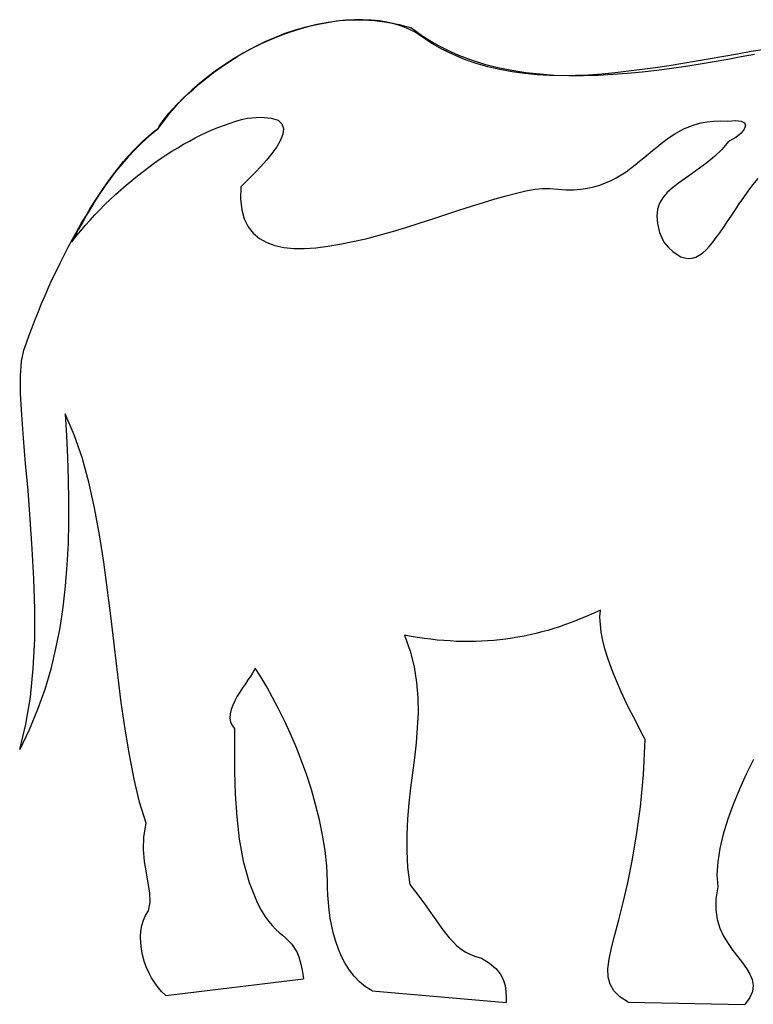
# Model space of a CAD drawing. Units: inches. Extents: x 386 to 107067, y -7 to 96314.
# Tile 7 of 10: x 101861.777 to 101863.94, y 96247.493 to 96250.395. Entities that reach past the tile are written whole.
import ezdxf

# ---------------------------------------------------------------- set-up
doc = ezdxf.new("R2010")
doc.units = ezdxf.units.IN
doc.layers.add('A-ELEV', color=7, linetype='Continuous', lineweight=25)
doc.layers.add('freecads.com', color=7, linetype='Continuous')

# ---------------------------------------------------------------- blocks, each defined once
blk = doc.blocks.new('elephant')
at = {"layer": 'freecads.com'}
for p, q in [((104457.3165, 95264.9791), (104457.3504, 95264.9835)), ((104457.3684, 95264.9845), (104457.3416, 95264.9818)), ((104457.3504, 95264.9835), (104457.3843, 95264.9856)), ((104457.3941, 95264.9862), (104457.3684, 95264.9845)), ((104457.3843, 95264.9856), (104457.4193, 95264.9856)), ((104457.4193, 95264.9862), (104457.3941, 95264.9862)), ((104457.4439, 95264.9851), (104457.4193, 95264.9862)), ((104457.4193, 95264.9856), (104457.4543, 95264.9835)), ((104457.4674, 95264.9829), (104457.4439, 95264.9851)), ((104457.4543, 95264.9835), (104457.4898, 95264.9791)), ((104457.4898, 95264.9791), (104457.4674, 95264.9829)), ((104457.1896, 95264.9463), (104457.2202, 95264.9567)), ((104457.2328, 95264.9583), (104457.2049, 95264.949)), ((104457.2202, 95264.9567), (104457.2514, 95264.9654)), ((104457.2601, 95264.966), (104457.2328, 95264.9583)), ((104457.2514, 95264.9654), (104457.2836, 95264.9731)), ((104457.288, 95264.9725), (104457.2601, 95264.966)), ((104457.2836, 95264.9731), (104457.3165, 95264.9791)), ((104457.3148, 95264.9774), (104457.288, 95264.9725)), ((104457.3416, 95264.9818), (104457.3148, 95264.9774)), ((104457.4898, 95264.9791), (104457.5259, 95264.972)), ((104457.5117, 95264.9742), (104457.4898, 95264.9791)), ((104457.5325, 95264.9676), (104457.5117, 95264.9742)), ((104457.5259, 95264.972), (104457.5625, 95264.9621)), ((104457.5522, 95264.9594), (104457.5325, 95264.9676)), ((104457.5708, 95264.9501), (104457.5522, 95264.9594)), ((104457.5625, 95264.9621), (104457.5954, 95264.9381)), ((104457.1491, 95264.9277), (104457.1212, 95264.9156)), ((104457.1311, 95264.9217), (104457.1595, 95264.9342)), ((104457.177, 95264.9392), (104457.1491, 95264.9277)), ((104457.1595, 95264.9342), (104457.1896, 95264.9463)), ((104457.2049, 95264.949), (104457.177, 95264.9392)), ((104457.5877, 95264.9392), (104457.5708, 95264.9501)), ((104457.6194, 95264.9184), (104457.5877, 95264.9392)), ((104457.5954, 95264.9381), (104457.6292, 95264.9167)), ((104457.0939, 95264.902), (104457.0665, 95264.8872)), ((104457.0758, 95264.8932), (104457.1032, 95264.908)), ((104457.1212, 95264.9156), (104457.0939, 95264.902)), ((104457.1032, 95264.908), (104457.1311, 95264.9217)), ((104457.6517, 95264.8998), (104457.6194, 95264.9184)), ((104457.6292, 95264.9167), (104457.6648, 95264.8981)), ((104457.685, 95264.8834), (104457.6517, 95264.8998)), ((104457.6648, 95264.8981), (104457.7009, 95264.8817)), ((104458.6048, 95264.8987), (104458.5644, 95264.8921)), ((104457.0398, 95264.8719), (104457.0135, 95264.8549)), ((104457.0255, 95264.8626), (104457.0501, 95264.8784)), ((104457.0665, 95264.8872), (104457.0398, 95264.8719)), ((104457.0501, 95264.8784), (104457.0758, 95264.8932)), ((104457.7184, 95264.8691), (104457.685, 95264.8834)), ((104457.7009, 95264.8817), (104457.7386, 95264.8675)), ((104457.7528, 95264.8571), (104457.7184, 95264.8691)), ((104457.7386, 95264.8675), (104457.7775, 95264.8555)), ((104458.443, 95264.8708), (104458.4025, 95264.8642)), ((104458.4834, 95264.8779), (104458.443, 95264.8708)), ((104458.4545, 95264.8631), (104458.4949, 95264.8702)), ((104458.5239, 95264.885), (104458.4834, 95264.8779)), ((104458.4949, 95264.8702), (104458.5348, 95264.8773)), ((104458.5644, 95264.8921), (104458.5239, 95264.885)), ((104458.5348, 95264.8773), (104458.5737, 95264.885)), ((104456.9878, 95264.8374), (104456.9626, 95264.8189)), ((104456.979, 95264.8303), (104457.0015, 95264.8467)), ((104457.0135, 95264.8549), (104456.9878, 95264.8374)), ((104457.0015, 95264.8467), (104457.0255, 95264.8626)), ((104457.7878, 95264.8473), (104457.7528, 95264.8571)), ((104457.7775, 95264.8555), (104457.8174, 95264.8451)), ((104457.8234, 95264.8391), (104457.7878, 95264.8473)), ((104457.8174, 95264.8451), (104457.8579, 95264.8374)), ((104457.8595, 95264.8325), (104457.8234, 95264.8391)), ((104457.8579, 95264.8374), (104457.8994, 95264.8309)), ((104458.2423, 95264.8391), (104458.2024, 95264.8342)), ((104458.2822, 95264.8446), (104458.2423, 95264.8391)), ((104458.2429, 95264.8325), (104458.286, 95264.8374)), ((104458.3221, 95264.8506), (104458.2822, 95264.8446)), ((104458.286, 95264.8374), (104458.3287, 95264.8435)), ((104458.3621, 95264.8571), (104458.3221, 95264.8506)), ((104458.3287, 95264.8435), (104458.3714, 95264.8495)), ((104458.4025, 95264.8642), (104458.3621, 95264.8571)), ((104458.3714, 95264.8495), (104458.4135, 95264.856)), ((104458.4135, 95264.856), (104458.4545, 95264.8631)), ((104456.9626, 95264.8189), (104456.938, 95264.7992)), ((104456.938, 95264.7981), (104456.9577, 95264.8139)), ((104456.9577, 95264.8139), (104456.979, 95264.8303)), ((104457.8961, 95264.8276), (104457.8595, 95264.8325)), ((104457.9328, 95264.8238), (104457.8961, 95264.8276)), ((104457.8994, 95264.8309), (104457.941, 95264.8265)), ((104457.9705, 95264.8221), (104457.9328, 95264.8238)), ((104457.941, 95264.8265), (104457.9836, 95264.8232)), ((104458.0082, 95264.821), (104457.9705, 95264.8221)), ((104457.9836, 95264.8232), (104458.0263, 95264.8221)), ((104458.0465, 95264.8216), (104458.0082, 95264.821)), ((104458.0263, 95264.8221), (104458.0695, 95264.8221)), ((104458.0848, 95264.8232), (104458.0465, 95264.8216)), ((104458.0695, 95264.8221), (104458.1127, 95264.8232)), ((104458.1236, 95264.826), (104458.0848, 95264.8232)), ((104458.1127, 95264.8232), (104458.1559, 95264.8254)), ((104458.163, 95264.8298), (104458.1236, 95264.826)), ((104458.1559, 95264.8254), (104458.1996, 95264.8287)), ((104458.2024, 95264.8342), (104458.163, 95264.8298)), ((104458.1996, 95264.8287), (104458.2429, 95264.8325)), ((104456.9019, 95264.7663), (104456.9194, 95264.7817)), ((104456.938, 95264.7992), (104456.9145, 95264.7784)), ((104456.9194, 95264.7817), (104456.938, 95264.7981)), ((104456.8915, 95264.757), (104456.8697, 95264.7341)), ((104456.8719, 95264.7368), (104456.8861, 95264.751)), ((104456.8861, 95264.751), (104456.9019, 95264.7663)), ((104456.9145, 95264.7784), (104456.8915, 95264.757)), ((104456.8472, 95264.7106), (104456.8587, 95264.7231)), ((104456.8697, 95264.7341), (104456.8489, 95264.7111)), ((104456.8587, 95264.7231), (104456.8719, 95264.7368)), ((104456.8489, 95264.7111), (104456.8297, 95264.6865)), ((104456.8297, 95264.6887), (104456.8379, 95264.6985)), ((104456.8379, 95264.6985), (104456.8472, 95264.7106)), ((104457.0447, 95264.6871), (104457.0616, 95264.692)), ((104457.0616, 95264.692), (104457.078, 95264.6958)), ((104457.078, 95264.6958), (104457.1185, 95264.6985)), ((104457.1185, 95264.6985), (104457.1486, 95264.6964)), ((104457.1486, 95264.6964), (104457.1688, 95264.6898)), ((104456.8013, 95264.6553), (104456.8161, 95264.6663)), ((104456.8297, 95264.6865), (104456.8111, 95264.6613)), ((104456.8161, 95264.6663), (104456.8188, 95264.6723)), ((104456.8188, 95264.6723), (104456.8232, 95264.6794)), ((104456.8232, 95264.6794), (104456.8297, 95264.6887)), ((104456.9768, 95264.6624), (104456.9938, 95264.6696)), ((104456.9938, 95264.6696), (104457.0108, 95264.6756)), ((104457.0108, 95264.6756), (104457.0277, 95264.6816)), ((104457.0277, 95264.6816), (104457.0447, 95264.6871)), ((104457.1688, 95264.6898), (104457.1803, 95264.6794)), ((104457.1803, 95264.6794), (104457.1852, 95264.6652)), ((104457.1852, 95264.6652), (104457.183, 95264.6493)), ((104458.3528, 95264.6581), (104458.3675, 95264.6652)), ((104458.3675, 95264.6652), (104458.3828, 95264.6717)), ((104458.3828, 95264.6717), (104458.3993, 95264.6778)), ((104458.3993, 95264.6778), (104458.4162, 95264.6821)), ((104458.4162, 95264.6821), (104458.4342, 95264.6854)), ((104458.4342, 95264.6854), (104458.4534, 95264.6876)), ((104458.4534, 95264.6876), (104458.473, 95264.6882)), ((104458.473, 95264.6882), (104458.4944, 95264.6871)), ((104458.4944, 95264.6871), (104458.5184, 95264.6892)), ((104458.5184, 95264.6892), (104458.5348, 95264.6876)), ((104458.5436, 95264.6635), (104458.5343, 95264.652)), ((104458.5348, 95264.6876), (104458.5447, 95264.6821)), ((104458.5474, 95264.6739), (104458.5436, 95264.6635)), ((104458.5447, 95264.6821), (104458.5474, 95264.6739)), ((104456.7887, 95264.6428), (104456.7669, 95264.6231)), ((104456.7718, 95264.6302), (104456.7865, 95264.6433)), ((104456.7865, 95264.6433), (104456.8013, 95264.6553)), ((104456.8111, 95264.6613), (104456.7887, 95264.6428)), ((104456.9074, 95264.6285), (104456.9249, 95264.6378)), ((104456.9249, 95264.6378), (104456.9424, 95264.6466)), ((104456.9424, 95264.6466), (104456.9593, 95264.6548)), ((104456.9593, 95264.6548), (104456.9768, 95264.6624)), ((104457.183, 95264.6493), (104457.1765, 95264.6313)), ((104458.3117, 95264.6313), (104458.3249, 95264.6411)), ((104458.3249, 95264.6411), (104458.3385, 95264.6499)), ((104458.3385, 95264.6499), (104458.3528, 95264.6581)), ((104458.5184, 95264.6395), (104458.4977, 95264.6274)), ((104458.5343, 95264.652), (104458.5184, 95264.6395)), ((104456.7422, 95264.6012), (104456.757, 95264.6159)), ((104456.7669, 95264.6231), (104456.7466, 95264.6028)), ((104456.757, 95264.6159), (104456.7718, 95264.6302)), ((104456.8554, 95264.5985), (104456.8729, 95264.6088)), ((104456.8729, 95264.6088), (104456.8905, 95264.6192)), ((104456.8905, 95264.6192), (104456.9074, 95264.6285)), ((104457.165, 95264.6116), (104457.1508, 95264.5919)), ((104457.1765, 95264.6313), (104457.165, 95264.6116)), ((104458.2729, 95264.6006), (104458.2855, 95264.611)), ((104458.2855, 95264.611), (104458.2986, 95264.6214)), ((104458.2986, 95264.6214), (104458.3117, 95264.6313)), ((104458.4977, 95264.6274), (104458.4774, 95264.6039)), ((104456.7269, 95264.5821), (104456.7083, 95264.5607)), ((104456.7133, 95264.5684), (104456.728, 95264.5848)), ((104456.7466, 95264.6028), (104456.7269, 95264.5821)), ((104456.728, 95264.5848), (104456.7422, 95264.6012)), ((104456.8046, 95264.564), (104456.8215, 95264.576)), ((104456.8215, 95264.576), (104456.8385, 95264.5875)), ((104456.8385, 95264.5875), (104456.8554, 95264.5985)), ((104457.1508, 95264.5919), (104457.1349, 95264.5722)), ((104458.2352, 95264.5689), (104458.2478, 95264.5793)), ((104458.2478, 95264.5793), (104458.2604, 95264.5903)), ((104458.2604, 95264.5903), (104458.2729, 95264.6006)), ((104458.4561, 95264.5831), (104458.4337, 95264.5646)), ((104458.4774, 95264.6039), (104458.4561, 95264.5831)), ((104456.6848, 95264.5317), (104456.699, 95264.5503)), ((104456.7083, 95264.5607), (104456.6908, 95264.5394)), ((104456.699, 95264.5503), (104456.7133, 95264.5684)), ((104456.7707, 95264.5389), (104456.7876, 95264.5514)), ((104456.7876, 95264.5514), (104456.8046, 95264.564)), ((104457.1179, 95264.5531), (104457.1015, 95264.5361)), ((104457.1349, 95264.5722), (104457.1179, 95264.5531)), ((104458.1953, 95264.5383), (104458.2089, 95264.5482)), ((104458.2089, 95264.5482), (104458.2221, 95264.5585)), ((104458.2221, 95264.5585), (104458.2352, 95264.5689)), ((104458.4118, 95264.5482), (104458.3905, 95264.5328)), ((104458.4337, 95264.5646), (104458.4118, 95264.5482)), ((104456.6701, 95264.5126), (104456.6848, 95264.5317)), ((104456.6908, 95264.5394), (104456.6739, 95264.5175)), ((104456.7379, 95264.5126), (104456.7543, 95264.5263)), ((104456.7543, 95264.5263), (104456.7707, 95264.5389)), ((104457.0862, 95264.5208), (104457.0736, 95264.5082)), ((104457.1015, 95264.5361), (104457.0862, 95264.5208)), ((104458.151, 95264.5126), (104458.1663, 95264.5203)), ((104458.1663, 95264.5203), (104458.181, 95264.529)), ((104458.181, 95264.529), (104458.1953, 95264.5383)), ((104458.3697, 95264.5186), (104458.35, 95264.5044)), ((104458.3905, 95264.5328), (104458.3697, 95264.5186)), ((104458.5693, 95264.4995), (104458.5846, 95264.5181)), ((104456.6422, 95264.4721), (104456.6564, 95264.4929)), ((104456.658, 95264.4956), (104456.6433, 95264.4738)), ((104456.6564, 95264.4929), (104456.6701, 95264.5126)), ((104456.6739, 95264.5175), (104456.658, 95264.4956)), ((104456.7056, 95264.4852), (104456.7215, 95264.4989)), ((104456.7215, 95264.4989), (104456.7379, 95264.5126)), ((104457.0594, 95264.494), (104457.0583, 95264.4579)), ((104457.0643, 95264.4989), (104457.0594, 95264.494)), ((104457.0736, 95264.5082), (104457.0643, 95264.4989)), ((104457.9257, 95264.4863), (104457.9486, 95264.4891)), ((104457.9486, 95264.4891), (104457.9689, 95264.4891)), ((104457.9689, 95264.4891), (104457.994, 95264.4863)), ((104458.0613, 95264.4863), (104458.081, 95264.4896)), ((104458.081, 95264.4896), (104458.1001, 95264.4935)), ((104458.1001, 95264.4935), (104458.1176, 95264.4989)), ((104458.1176, 95264.4989), (104458.1346, 95264.5055)), ((104458.1346, 95264.5055), (104458.151, 95264.5126)), ((104458.3325, 95264.4907), (104458.3167, 95264.4765)), ((104458.35, 95264.5044), (104458.3325, 95264.4907)), ((104458.5551, 95264.4809), (104458.5693, 95264.4995)), ((104456.6285, 95264.4513), (104456.6422, 95264.4721)), ((104456.6433, 95264.4738), (104456.6291, 95264.4519)), ((104456.6739, 95264.4563), (104456.6897, 95264.471)), ((104456.6897, 95264.471), (104456.7056, 95264.4852)), ((104457.8092, 95264.4579), (104457.8415, 95264.4672)), ((104457.8415, 95264.4672), (104457.8721, 95264.4754)), ((104457.8721, 95264.4754), (104457.8999, 95264.482)), ((104457.8999, 95264.482), (104457.9257, 95264.4863)), ((104457.994, 95264.4863), (104458.0175, 95264.4847)), ((104458.0175, 95264.4847), (104458.0399, 95264.4847)), ((104458.0399, 95264.4847), (104458.0613, 95264.4863)), ((104458.3035, 95264.4617), (104458.2937, 95264.4459)), ((104458.3167, 95264.4765), (104458.3035, 95264.4617)), ((104458.5288, 95264.4437), (104458.542, 95264.4623)), ((104458.542, 95264.4623), (104458.5551, 95264.4809)), ((104456.6148, 95264.4295), (104456.6285, 95264.4513)), ((104456.6291, 95264.4519), (104456.6159, 95264.43)), ((104456.6438, 95264.4262), (104456.6586, 95264.4415)), ((104456.6586, 95264.4415), (104456.6739, 95264.4563)), ((104457.0583, 95264.4579), (104457.0622, 95264.4262)), ((104457.702, 95264.4246), (104457.7392, 95264.4366)), ((104457.7392, 95264.4366), (104457.7747, 95264.4475)), ((104457.7747, 95264.4475), (104457.8092, 95264.4579)), ((104458.2937, 95264.4459), (104458.2877, 95264.4278)), ((104458.5168, 95264.4251), (104458.5288, 95264.4437)), ((104456.5886, 95264.3852), (104456.6017, 95264.4076)), ((104456.6033, 95264.4092), (104456.5919, 95264.3885)), ((104456.6017, 95264.4076), (104456.6148, 95264.4295)), ((104456.6159, 95264.43), (104456.6033, 95264.4092)), ((104456.6148, 95264.3956), (104456.6291, 95264.4109)), ((104456.6291, 95264.4109), (104456.6438, 95264.4262)), ((104457.0622, 95264.4262), (104457.0693, 95264.3989)), ((104457.6249, 95264.3994), (104457.6637, 95264.412)), ((104457.6637, 95264.412), (104457.702, 95264.4246)), ((104458.2877, 95264.4278), (104458.2855, 95264.4076)), ((104458.2855, 95264.4076), (104458.2877, 95264.3852)), ((104458.4933, 95264.3907), (104458.5048, 95264.4076)), ((104458.5048, 95264.4076), (104458.5168, 95264.4251)), ((104456.5754, 95264.3622), (104456.5886, 95264.3852)), ((104456.5919, 95264.3885), (104456.5809, 95264.3688)), ((104456.5869, 95264.3638), (104456.6006, 95264.3797)), ((104456.6006, 95264.3797), (104456.6148, 95264.3956)), ((104457.0693, 95264.3989), (104457.0807, 95264.3759)), ((104457.0807, 95264.3759), (104457.0955, 95264.3567)), ((104457.5062, 95264.3622), (104457.5461, 95264.3742)), ((104457.5461, 95264.3742), (104457.5855, 95264.3868)), ((104457.5855, 95264.3868), (104457.6249, 95264.3994)), ((104458.2877, 95264.3852), (104458.2942, 95264.3595)), ((104458.4714, 95264.3584), (104458.4823, 95264.3742)), ((104458.4823, 95264.3742), (104458.4933, 95264.3907)), ((104456.5705, 95264.3496), (104456.5607, 95264.3316)), ((104456.5607, 95264.3316), (104456.5738, 95264.348)), ((104456.5629, 95264.3392), (104456.5754, 95264.3622)), ((104456.5809, 95264.3688), (104456.5705, 95264.3496)), ((104456.5738, 95264.348), (104456.5869, 95264.3638)), ((104457.0955, 95264.3567), (104457.1141, 95264.3414)), ((104457.4275, 95264.3409), (104457.4668, 95264.3513)), ((104457.4668, 95264.3513), (104457.5062, 95264.3622)), ((104458.2942, 95264.3595), (104458.3068, 95264.3305)), ((104458.4512, 95264.3305), (104458.461, 95264.3442)), ((104458.461, 95264.3442), (104458.4714, 95264.3584)), ((104456.5383, 95264.2922), (104456.5503, 95264.3157)), ((104456.5503, 95264.3157), (104456.5629, 95264.3392)), ((104457.1141, 95264.3414), (104457.1354, 95264.3294)), ((104457.1354, 95264.3294), (104457.1595, 95264.3212)), ((104457.1595, 95264.3212), (104457.1863, 95264.3152)), ((104457.1863, 95264.3152), (104457.2158, 95264.3124)), ((104457.2804, 95264.3141), (104457.3154, 95264.3185)), ((104457.3154, 95264.3185), (104457.3514, 95264.3245)), ((104457.3514, 95264.3245), (104457.3892, 95264.3321)), ((104457.3892, 95264.3321), (104457.4275, 95264.3409)), ((104458.3068, 95264.3305), (104458.3205, 95264.3152)), ((104458.3205, 95264.3152), (104458.3331, 95264.3032)), ((104458.431, 95264.3081), (104458.4408, 95264.3185)), ((104458.4408, 95264.3185), (104458.4512, 95264.3305)), ((104456.5262, 95264.2687), (104456.5383, 95264.2922)), ((104457.2158, 95264.3124), (104457.247, 95264.3124)), ((104457.247, 95264.3124), (104457.2804, 95264.3141)), ((104458.3331, 95264.3032), (104458.3457, 95264.2939)), ((104458.3457, 95264.2939), (104458.3571, 95264.2878)), ((104458.3571, 95264.2878), (104458.3686, 95264.284)), ((104458.3905, 95264.2835), (104458.4009, 95264.2868)), ((104458.4009, 95264.2868), (104458.4107, 95264.2922)), ((104458.4107, 95264.2922), (104458.4211, 95264.2993)), ((104458.4211, 95264.2993), (104458.431, 95264.3081)), ((104456.5148, 95264.2446), (104456.5262, 95264.2687)), ((104458.3686, 95264.284), (104458.3796, 95264.2824)), ((104458.3796, 95264.2824), (104458.3905, 95264.2835)), ((104456.5033, 95264.2211), (104456.5148, 95264.2446)), ((104456.4923, 95264.197), (104456.5033, 95264.2211)), ((104456.4716, 95264.1495), (104456.4819, 95264.173)), ((104456.4819, 95264.173), (104456.4923, 95264.197)), ((104456.4623, 95264.126), (104456.4716, 95264.1495)), ((104456.4524, 95264.1024), (104456.4623, 95264.126)), ((104456.4437, 95264.0795), (104456.4524, 95264.1024)), ((104456.4272, 95264.0341), (104456.4354, 95264.0565)), ((104456.4354, 95264.0565), (104456.4437, 95264.0795)), ((104456.4196, 95264.0122), (104456.4272, 95264.0341)), ((104456.4125, 95263.98), (104456.4196, 95264.0122)), ((104456.4097, 95263.9367), (104456.4125, 95263.98)), ((104456.4097, 95263.8837), (104456.4097, 95263.9367)), ((104456.413, 95263.8219), (104456.4097, 95263.8837)), ((104456.4179, 95263.753), (104456.413, 95263.8219)), ((104456.5678, 95263.7629), (104456.5415, 95263.8246)), ((104456.5415, 95263.8246), (104456.5448, 95263.7601)), ((104456.4245, 95263.6781), (104456.4179, 95263.753)), ((104456.5448, 95263.7601), (104456.5481, 95263.6961)), ((104456.5908, 95263.6956), (104456.5678, 95263.7629)), ((104456.4316, 95263.5983), (104456.4245, 95263.6781)), ((104456.5481, 95263.6961), (104456.5497, 95263.6322)), ((104456.6105, 95263.6234), (104456.5908, 95263.6956)), ((104456.5497, 95263.6322), (104456.5514, 95263.5687)), ((104456.6274, 95263.5474), (104456.6105, 95263.6234)), ((104456.4382, 95263.514), (104456.4316, 95263.5983)), ((104456.5514, 95263.5687), (104456.5514, 95263.5053)), ((104456.6422, 95263.4686), (104456.6274, 95263.5474)), ((104456.4442, 95263.4271), (104456.4382, 95263.514)), ((104456.5514, 95263.5053), (104456.5497, 95263.4424)), ((104456.6547, 95263.3877), (104456.6422, 95263.4686)), ((104456.4491, 95263.3385), (104456.4442, 95263.4271)), ((104456.5497, 95263.4424), (104456.5465, 95263.3795)), ((104456.6662, 95263.3046), (104456.6547, 95263.3877)), ((104456.5465, 95263.3795), (104456.5415, 95263.3172)), ((104456.4513, 95263.2494), (104456.4491, 95263.3385)), ((104456.5415, 95263.3172), (104456.5344, 95263.2554)), ((104456.6766, 95263.2215), (104456.6662, 95263.3046)), ((104456.4513, 95263.1608), (104456.4513, 95263.2494)), ((104456.5344, 95263.2554), (104456.5251, 95263.1936)), ((104458.1193, 95263.2466), (104458.1023, 95263.2384)), ((104458.1182, 95263.2258), (104458.1193, 95263.2466)), ((104456.6865, 95263.1378), (104456.6766, 95263.2215)), ((104458.0509, 95263.2165), (104458.0334, 95263.2094)), ((104458.0678, 95263.2231), (104458.0509, 95263.2165)), ((104458.0848, 95263.2308), (104458.0678, 95263.2231)), ((104458.1023, 95263.2384), (104458.0848, 95263.2308)), ((104458.1193, 95263.204), (104458.1182, 95263.2258)), ((104456.5251, 95263.1936), (104456.5131, 95263.1329)), ((104457.9645, 95263.1865), (104457.947, 95263.1821)), ((104457.982, 95263.1919), (104457.9645, 95263.1865)), ((104457.9989, 95263.1974), (104457.982, 95263.1919)), ((104458.0164, 95263.2034), (104457.9989, 95263.1974)), ((104458.0334, 95263.2094), (104458.0164, 95263.2034)), ((104458.122, 95263.181), (104458.1193, 95263.204)), ((104456.4469, 95263.0738), (104456.4513, 95263.1608)), ((104457.5615, 95263.169), (104457.5418, 95263.1728)), ((104457.5418, 95263.1728), (104457.5582, 95263.1252)), ((104457.5806, 95263.1657), (104457.5615, 95263.169)), ((104457.6003, 95263.163), (104457.5806, 95263.1657)), ((104457.6194, 95263.1602), (104457.6003, 95263.163)), ((104457.6385, 95263.158), (104457.6194, 95263.1602)), ((104457.6577, 95263.1564), (104457.6385, 95263.158)), ((104457.6763, 95263.1553), (104457.6577, 95263.1564)), ((104457.6949, 95263.1542), (104457.6763, 95263.1553)), ((104457.7135, 95263.1537), (104457.6949, 95263.1542)), ((104457.7687, 95263.1548), (104457.7507, 95263.1537)), ((104457.7868, 95263.1553), (104457.7687, 95263.1548)), ((104457.8048, 95263.157), (104457.7868, 95263.1553)), ((104457.8229, 95263.1586), (104457.8048, 95263.157)), ((104457.8409, 95263.1608), (104457.8229, 95263.1586)), ((104457.859, 95263.1635), (104457.8409, 95263.1608)), ((104457.8764, 95263.1662), (104457.859, 95263.1635)), ((104457.8945, 95263.1695), (104457.8764, 95263.1662)), ((104457.912, 95263.1734), (104457.8945, 95263.1695)), ((104457.9295, 95263.1772), (104457.912, 95263.1734)), ((104457.947, 95263.1821), (104457.9295, 95263.1772)), ((104458.1264, 95263.157), (104458.122, 95263.181)), ((104458.1329, 95263.1323), (104458.1264, 95263.157)), ((104456.5131, 95263.1329), (104456.4984, 95263.0722)), ((104456.6968, 95263.0552), (104456.6865, 95263.1378)), ((104457.5582, 95263.1252), (104457.5702, 95263.0787)), ((104457.7321, 95263.1537), (104457.7135, 95263.1537)), ((104457.7507, 95263.1537), (104457.7321, 95263.1537)), ((104458.1406, 95263.1077), (104458.1329, 95263.1323)), ((104458.1493, 95263.082), (104458.1406, 95263.1077)), ((104456.4387, 95262.9901), (104456.4469, 95263.0738)), ((104456.4984, 95263.0722), (104456.4808, 95263.012)), ((104457.0982, 95263.0689), (104457.0933, 95263.0607)), ((104457.1015, 95263.0754), (104457.0982, 95263.0689)), ((104457.1179, 95263.0492), (104457.1015, 95263.0754)), ((104457.5702, 95263.0787), (104457.5773, 95263.0334)), ((104458.1592, 95263.0569), (104458.1493, 95263.082)), ((104456.7067, 95262.9743), (104456.6968, 95263.0552)), ((104457.0802, 95263.0405), (104457.0725, 95263.0295)), ((104457.0873, 95263.0508), (104457.0802, 95263.0405)), ((104457.0933, 95263.0607), (104457.0873, 95263.0508)), ((104457.1354, 95263.0202), (104457.1179, 95263.0492)), ((104458.1696, 95263.0312), (104458.1592, 95263.0569)), ((104456.4808, 95263.012), (104456.4595, 95262.953)), ((104457.0643, 95263.0175), (104457.0561, 95263.0049)), ((104457.0725, 95263.0295), (104457.0643, 95263.0175)), ((104457.1529, 95262.9891), (104457.1354, 95263.0202)), ((104457.5773, 95263.0334), (104457.5811, 95262.988)), ((104458.181, 95263.0055), (104458.1696, 95263.0312)), ((104456.4256, 95262.9103), (104456.4387, 95262.9901)), ((104457.0485, 95262.9923), (104457.0414, 95262.9792)), ((104457.0561, 95263.0049), (104457.0485, 95262.9923)), ((104457.1704, 95262.9551), (104457.1529, 95262.9891)), ((104457.5811, 95262.988), (104457.5817, 95262.9437)), ((104458.1925, 95262.9803), (104458.181, 95263.0055)), ((104458.2046, 95262.9557), (104458.1925, 95262.9803)), ((104456.4595, 95262.953), (104456.4354, 95262.8939)), ((104456.7182, 95262.895), (104456.7067, 95262.9743)), ((104457.031, 95262.953), (104457.0277, 95262.9404)), ((104457.0354, 95262.9661), (104457.031, 95262.953)), ((104457.0414, 95262.9792), (104457.0354, 95262.9661)), ((104457.1879, 95262.9196), (104457.1704, 95262.9551)), ((104458.2166, 95262.9316), (104458.2046, 95262.9557)), ((104457.0277, 95262.9404), (104457.0272, 95262.9283)), ((104457.0272, 95262.9283), (104457.0288, 95262.9174)), ((104457.5817, 95262.9437), (104457.5795, 95262.8994)), ((104458.2286, 95262.9087), (104458.2166, 95262.9316)), ((104456.407, 95262.8359), (104456.4256, 95262.9103)), ((104456.4354, 95262.8939), (104456.407, 95262.8359)), ((104456.7308, 95262.8195), (104456.7182, 95262.895)), ((104457.0288, 95262.9174), (104457.0332, 95262.9065)), ((104457.0332, 95262.9065), (104457.0403, 95262.8972)), ((104457.0403, 95262.8972), (104457.0403, 95262.8348)), ((104457.2054, 95262.8819), (104457.1879, 95262.9196)), ((104457.5795, 95262.8994), (104457.5762, 95262.8556)), ((104458.2401, 95262.8863), (104458.2286, 95262.9087)), ((104457.2224, 95262.843), (104457.2054, 95262.8819)), ((104458.2516, 95262.8649), (104458.2401, 95262.8863)), ((104458.2461, 95262.7605), (104458.2516, 95262.8649)), ((104457.0403, 95262.8348), (104457.0408, 95262.7703)), ((104457.2382, 95262.802), (104457.2224, 95262.843)), ((104457.5762, 95262.8556), (104457.5713, 95262.8113)), ((104456.7444, 95262.7479), (104456.7308, 95262.8195)), ((104457.5713, 95262.8113), (104457.5653, 95262.767)), ((104458.571, 95262.8058), (104458.5496, 95262.7627)), ((104457.2536, 95262.7599), (104457.2382, 95262.802)), ((104456.7608, 95262.6806), (104456.7444, 95262.7479)), ((104457.0408, 95262.7703), (104457.0425, 95262.7041)), ((104457.2672, 95262.7173), (104457.2536, 95262.7599)), ((104457.5653, 95262.767), (104457.5598, 95262.7227)), ((104458.2374, 95262.6664), (104458.2461, 95262.7605)), ((104458.5496, 95262.7627), (104458.5294, 95262.7184)), ((104457.5598, 95262.7227), (104457.5543, 95262.6773)), ((104457.0425, 95262.7041), (104457.0469, 95262.6374)), ((104457.2798, 95262.673), (104457.2672, 95262.7173)), ((104458.5294, 95262.7184), (104458.5113, 95262.6735)), ((104456.78, 95262.6188), (104456.7608, 95262.6806)), ((104457.2913, 95262.6287), (104457.2798, 95262.673)), ((104457.5543, 95262.6773), (104457.5505, 95262.6314)), ((104458.2259, 95262.5827), (104458.2374, 95262.6664)), ((104458.5113, 95262.6735), (104458.4955, 95262.6298)), ((104457.0469, 95262.6374), (104457.0545, 95262.5712)), ((104456.7729, 95262.5784), (104456.78, 95262.6188)), ((104457.3001, 95262.5833), (104457.2913, 95262.6287)), ((104457.5505, 95262.6314), (104457.5483, 95262.5849)), ((104458.4955, 95262.6298), (104458.4818, 95262.586)), ((104456.7718, 95262.5406), (104456.7729, 95262.5784)), ((104457.3077, 95262.5379), (104457.3001, 95262.5833)), ((104457.5483, 95262.5849), (104457.5483, 95262.5368)), ((104458.2133, 95262.5078), (104458.2259, 95262.5827)), ((104458.4818, 95262.586), (104458.472, 95262.5439)), ((104457.0545, 95262.5712), (104457.0665, 95262.5062)), ((104456.7751, 95262.5051), (104456.7718, 95262.5406)), ((104457.3126, 95262.4925), (104457.3077, 95262.5379)), ((104457.5483, 95262.5368), (104457.5511, 95262.4876)), ((104458.472, 95262.5439), (104458.4654, 95262.504)), ((104456.7805, 95262.4723), (104456.7751, 95262.5051)), ((104457.0665, 95262.5062), (104457.084, 95262.4433)), ((104457.3148, 95262.4471), (104457.3126, 95262.4925)), ((104457.5511, 95262.4876), (104457.5576, 95262.4373)), ((104458.2002, 95262.4422), (104458.2133, 95262.5078)), ((104458.4654, 95262.504), (104458.4632, 95262.4663)), ((104456.786, 95262.4416), (104456.7805, 95262.4723)), ((104458.4632, 95262.4663), (104458.4654, 95262.4312)), ((104456.7904, 95262.4127), (104456.786, 95262.4416)), ((104457.084, 95262.4433), (104457.1075, 95262.3842)), ((104457.3148, 95262.4274), (104457.3148, 95262.4471)), ((104457.5576, 95262.4373), (104457.5746, 95262.4159)), ((104458.1865, 95262.3842), (104458.2002, 95262.4422)), ((104458.4654, 95262.4312), (104458.4599, 95262.3957)), ((104456.7915, 95262.3853), (104456.7904, 95262.4127)), ((104457.3159, 95262.4061), (104457.3148, 95262.4274)), ((104457.3176, 95262.3842), (104457.3159, 95262.4061)), ((104457.5746, 95262.4159), (104457.5899, 95262.3957)), ((104456.7865, 95262.3596), (104456.7915, 95262.3853)), ((104457.1075, 95262.3842), (104457.119, 95262.3623)), ((104457.3197, 95262.3618), (104457.3176, 95262.3842)), ((104457.5899, 95262.3957), (104457.6041, 95262.3766)), ((104457.6041, 95262.3766), (104457.6167, 95262.358)), ((104458.1734, 95262.3334), (104458.1865, 95262.3842)), ((104458.4599, 95262.3957), (104458.4594, 95262.364)), ((104456.7718, 95262.3323), (104456.7783, 95262.3465)), ((104456.7783, 95262.3465), (104456.7865, 95262.3596)), ((104457.119, 95262.3623), (104457.13, 95262.3443)), ((104457.13, 95262.3443), (104457.1415, 95262.329)), ((104457.323, 95262.3388), (104457.3197, 95262.3618)), ((104457.6167, 95262.358), (104457.6292, 95262.3405)), ((104458.4594, 95262.364), (104458.4638, 95262.335)), ((104456.7647, 95262.3005), (104456.7674, 95262.317)), ((104456.7674, 95262.317), (104456.7718, 95262.3323)), ((104457.1415, 95262.329), (104457.1519, 95262.3164)), ((104457.1519, 95262.3164), (104457.1628, 95262.3055)), ((104457.3274, 95262.3153), (104457.323, 95262.3388)), ((104457.3329, 95262.2923), (104457.3274, 95262.3153)), ((104457.6292, 95262.3405), (104457.6407, 95262.3241)), ((104457.6407, 95262.3241), (104457.6517, 95262.3082)), ((104458.1619, 95262.2896), (104458.1734, 95262.3334)), ((104458.4638, 95262.335), (104458.472, 95262.3088)), ((104456.7636, 95262.283), (104456.7647, 95262.3005)), ((104457.1628, 95262.3055), (104457.1726, 95262.2962)), ((104457.1726, 95262.2962), (104457.1825, 95262.288)), ((104457.1825, 95262.288), (104457.1923, 95262.2798)), ((104457.3394, 95262.2694), (104457.3329, 95262.2923)), ((104457.6517, 95262.3082), (104457.6626, 95262.294)), ((104457.6626, 95262.294), (104457.6736, 95262.2803)), ((104458.1521, 95262.2513), (104458.1619, 95262.2896)), ((104458.472, 95262.3088), (104458.4829, 95262.2852)), ((104458.4829, 95262.2852), (104458.496, 95262.2634)), ((104456.7641, 95262.2655), (104456.7636, 95262.283)), ((104456.7658, 95262.2475), (104456.7641, 95262.2655)), ((104457.1923, 95262.2798), (104457.2011, 95262.271)), ((104457.2011, 95262.271), (104457.2093, 95262.2623)), ((104457.2093, 95262.2623), (104457.2169, 95262.2513)), ((104457.3476, 95262.247), (104457.3394, 95262.2694)), ((104457.6736, 95262.2803), (104457.685, 95262.2683)), ((104457.685, 95262.2683), (104457.6965, 95262.2573)), ((104457.6965, 95262.2573), (104457.7086, 95262.247)), ((104458.496, 95262.2634), (104458.5102, 95262.2431)), ((104456.7696, 95262.23), (104456.7658, 95262.2475)), ((104456.774, 95262.212), (104456.7696, 95262.23)), ((104457.2169, 95262.2513), (104457.224, 95262.2393)), ((104457.224, 95262.2393), (104457.23, 95262.2245)), ((104457.3564, 95262.2256), (104457.3476, 95262.247)), ((104457.3673, 95262.2049), (104457.3564, 95262.2256)), ((104457.7086, 95262.247), (104457.7222, 95262.2382)), ((104457.7222, 95262.2382), (104457.7364, 95262.2311)), ((104457.7364, 95262.2311), (104457.7518, 95262.2251)), ((104458.1455, 95262.218), (104458.1521, 95262.2513)), ((104458.5102, 95262.2431), (104458.5245, 95262.2245)), ((104456.78, 95262.195), (104456.774, 95262.212)), ((104457.23, 95262.2245), (104457.2355, 95262.2065)), ((104457.2355, 95262.2065), (104457.2399, 95262.1852)), ((104457.3799, 95262.1852), (104457.3673, 95262.2049)), ((104457.7518, 95262.2251), (104457.7687, 95262.2202)), ((104457.7687, 95262.2202), (104457.7928, 95262.206)), ((104457.7928, 95262.206), (104457.8108, 95262.1901)), ((104458.1417, 95262.1895), (104458.1455, 95262.218)), ((104458.5245, 95262.2245), (104458.5381, 95262.207)), ((104458.5381, 95262.207), (104458.5507, 95262.1901)), ((104456.7876, 95262.1781), (104456.78, 95262.195)), ((104456.7958, 95262.1622), (104456.7876, 95262.1781)), ((104457.2399, 95262.1852), (104457.2437, 95262.1595)), ((104457.3936, 95262.1671), (104457.3799, 95262.1852)), ((104457.8108, 95262.1901), (104457.8239, 95262.1742)), ((104457.8239, 95262.1742), (104457.8327, 95262.1573)), ((104458.1422, 95262.1649), (104458.1417, 95262.1895)), ((104458.5507, 95262.1901), (104458.5606, 95262.1737)), ((104458.5606, 95262.1737), (104458.5671, 95262.1573)), ((104456.8051, 95262.1474), (104456.7958, 95262.1622)), ((104456.815, 95262.1337), (104456.8051, 95262.1474)), ((104456.8379, 95262.1108), (104457.2437, 95262.1595)), ((104457.4094, 95262.1513), (104457.3936, 95262.1671)), ((104457.4269, 95262.1365), (104457.4094, 95262.1513)), ((104457.8327, 95262.1573), (104457.8382, 95262.1398)), ((104457.8382, 95262.1398), (104457.8404, 95262.1228)), ((104458.1482, 95262.1436), (104458.1422, 95262.1649)), ((104458.1592, 95262.1244), (104458.1482, 95262.1436)), ((104458.5671, 95262.1573), (104458.5699, 95262.1403)), ((104458.5699, 95262.1403), (104458.5677, 95262.1228)), ((104456.8259, 95262.1212), (104456.815, 95262.1337)), ((104456.8379, 95262.1108), (104456.8259, 95262.1212)), ((104457.4466, 95262.1244), (104457.4269, 95262.1365)), ((104457.4466, 95262.1244), (104457.8415, 95262.0895)), ((104457.8404, 95262.1228), (104457.8415, 95262.1059)), ((104458.1767, 95262.107), (104458.1592, 95262.1244)), ((104458.5677, 95262.1228), (104458.56, 95262.1042)), ((104457.8415, 95262.1059), (104457.8415, 95262.0895)), ((104458.2013, 95262.0911), (104458.1767, 95262.107)), ((104458.2013, 95262.0911), (104458.5452, 95262.0845)), ((104458.56, 95262.1042), (104458.5452, 95262.0845))]:
    blk.add_line(p, q, dxfattribs=at)

msp = doc.modelspace()

# ---------------------------------------------------------------- block references
at = {"layer": 'A-ELEV'}
msp.add_blockref('elephant', (-2594.6305, 985.4087), dxfattribs=at)

doc.saveas('drawing.dxf')
